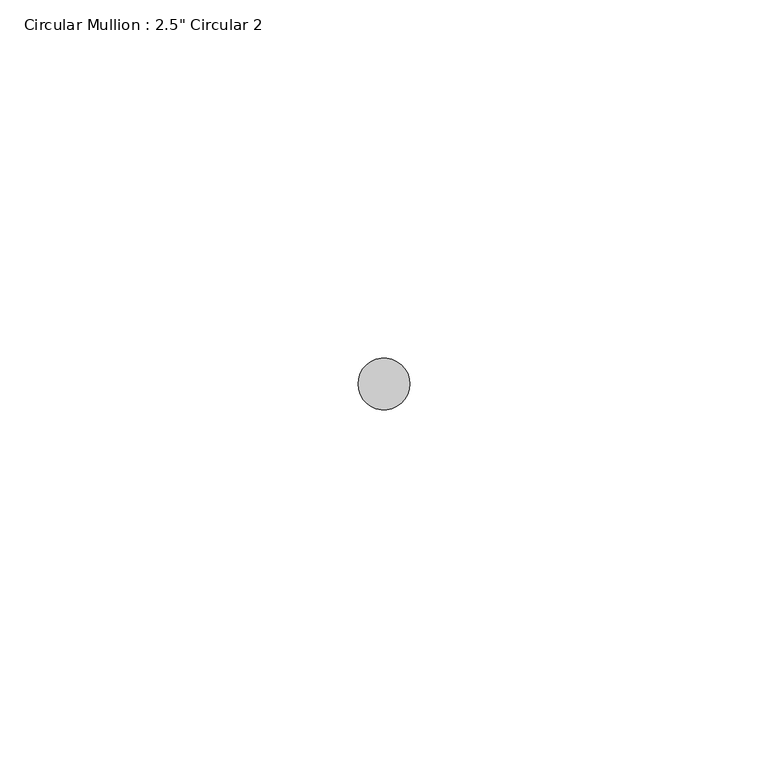
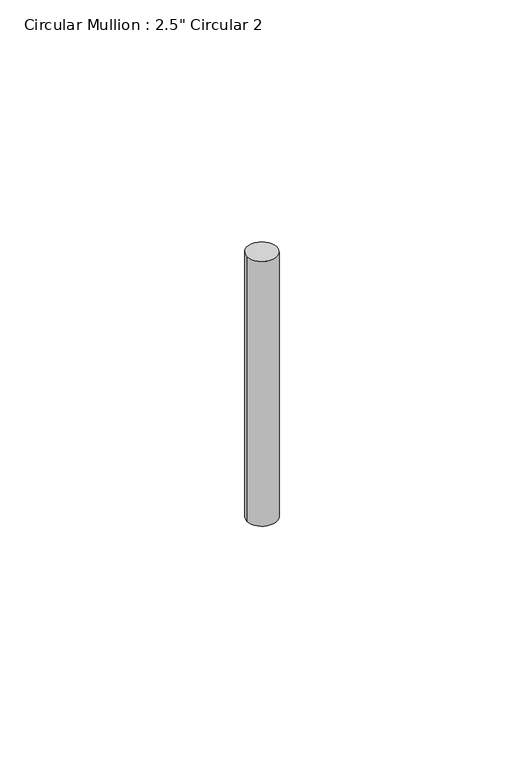
"""IFC4 building model written with IfcOpenShell, lengths in millimetres: member geometry."""

from ifc_helpers import new_model, si_unit, point, frame, frame_2d, origin, place, context, project, spatial, circle_curve, trimmed, segment, composite_curve, outline, extrude, source, transform, mapped, element, save


def member_3b441234(model_context):
    return source(origin(), model_context, "Body", "SweptSolid", [
        extrude(outline(composite_curve([segment(trimmed(circle_curve(frame_2d((-3.6195, 0.0)), 3.6195), [point((0.0, 0.0))], [point((-7.239, 0.0))], False, "CARTESIAN"), True, "CONTINUOUS"), segment(trimmed(circle_curve(frame_2d((-3.6195, 0.0)), 3.6195), [point((-7.239, 0.0))], [point((0.0, 0.0))], False, "CARTESIAN"), True, "CONTINUOUS")], self_intersect=False)), frame((0.0, 0.0, -67.7333333), z_axis=(0.0, 0.0, 1.0), x_axis=(1.0, 0.0, 0.0)), (0.0, 0.0, 1.0), 67.7333333),
    ])


if __name__ == "__main__":
    model = new_model("IFC4")
    model_context = context("Model", 3, world=origin())
    ifc_project = project(units=[si_unit("LENGTHUNIT", "METRE", prefix="MILLI")], contexts=[model_context])
    site = spatial("IfcSite", under=ifc_project)
    building = spatial("IfcBuilding", under=site)
    placement = place(None, origin())
    member_shape = member_3b441234(model_context)
    element("IfcMember", 1, ObjectType="Circular Mullion : 2.5\" Circular 2", at=placement, inside=building, context=model_context, shape_type="MappedRepresentation", body=[
        mapped(member_shape, transform((0.0, 0.0, 0.0), x_axis=(1.0, 0.0, 0.0), y_axis=(0.0, 1.0, 0.0), z_axis=(0.0, 0.0, 1.0))),
    ])
    save(model, "model.ifc")

# Revit data of these elements
# Type "Circular Mullion : 2.5\" Circular 2"
#   built-in parameter 1007350 = 0.011875 (stored number, unit not read)
# Element 1 (IfcMember, "Circular Mullion : 2.5\" Circular 2")
#   Materials on its faces: "Aluminum"
# Materials
#   "Aluminum": class "Metal", colour RGB 247 247 247, transparency 0, Description = "Aluminum 6061", Cost = 0
